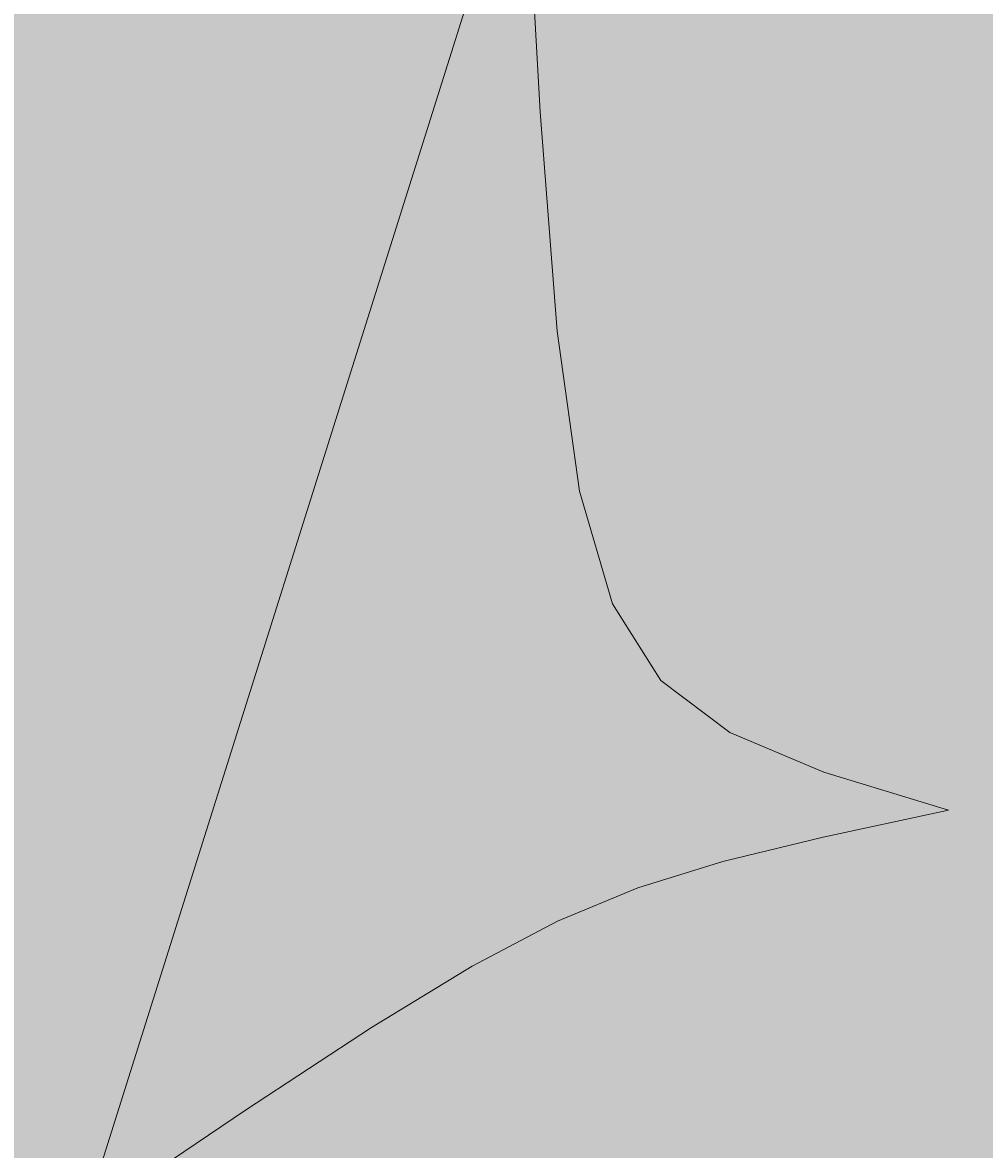
# Model space of a CAD drawing. Units: millimetres. Extents: x 27017497 to 27018854, y 7058029 to 7059154.
# Tile 84 of 91: x 27018341 to 27018362, y 7058530 to 7058555. Entities that reach past the tile are written whole.
import ezdxf

# ---------------------------------------------------------------- set-up
doc = ezdxf.new("R2010")
doc.units = ezdxf.units.MM
doc.layers.add('A-ANNO-DIMS', color=2, linetype='Continuous', lineweight=18)
doc.layers.add('A-FURN', color=8, linetype='Continuous', lineweight=18)
doc.layers.add('A-FURN-PATT', color=177, linetype='Continuous', lineweight=13, true_color=0x293189)
doc.styles.get("Standard").update_dxf_attribs({"font": 'arial.ttf'})
doc.dimstyles.get("Standard").update_dxf_attribs({"dimtxt": 0.18, "dimasz": 0.18, "dimexe": 0.18, "dimexo": 0.0625, "dimgap": 0.09, "dimtad": 0, "dimtih": 1, "dimtoh": 1, "dimdec": 4, "dimzin": 0, "dimdsep": 46, "dimtxsty": 'Standard', "dimcen": 0.09, "dimadec": 0, "dimazin": 0, "dimtfac": 1, "dimtdec": 4, "dimtofl": 0, "dimtmove": 0, "dimatfit": 3, "dimfxl": 1, "dimtolj": 1, "dimtzin": 0, "dimarcsym": 0})

# ---------------------------------------------------------------- blocks, each defined once
blk = doc.blocks.new('CAMMAT')
blk.add_line((0.05354, -0.5623), (-0.73116, -0.80928))
for points in [[(-0.17613, -1.04763), (-0.161, -0.97721), (-0.14737, -0.92096), (-0.13256, -0.87318), (-0.11386, -0.82818), (-0.0886, -0.78028), (-0.05407, -0.7238), (-0.00759, -0.65303), (0.05354, -0.5623)], [(-0.73116, -0.80928), (-0.56827, -0.81849), (-0.4451, -0.82799), (-0.35515, -0.84058), (-0.29193, -0.85906), (-0.24892, -0.8862), (-0.21962, -0.92482), (-0.19752, -0.9777), (-0.17613, -1.04763)]]:
    blk.add_lwpolyline(points)
blk = doc.blocks.new('*D48')
at = {"layer": 'A-ANNO-DIMS', "color": 0, "lineweight": -2, "transparency": 16777216}
for p, q in [((27018463.498, 7058622.912), (27017497.536, 7058622.912)), ((27017497.716, 7058622.732), (27017497.716, 7058357.753)), ((27017497.716, 7058092.41), (27017497.716, 7058357.389)), ((27018555.129, 7058092.23), (27017497.536, 7058092.23))]:
    blk.add_line(p, q, dxfattribs=at)
at = {"layer": 'A-ANNO-DIMS', "color": 0, "transparency": 16777216}
for points in [[(27017497.686, 7058622.732), (27017497.746, 7058622.732), (27017497.716, 7058622.912)], [(27017497.686, 7058092.41), (27017497.746, 7058092.41), (27017497.716, 7058092.23)]]:
    blk.add_solid(points, dxfattribs=at)
at = {"layer": 'Defpoints', "color": 0, "transparency": 16777216}
for p in [(27018463.561, 7058622.912), (27017497.716, 7058092.23), (27018555.192, 7058092.23)]:
    blk.add_point(p, dxfattribs=at)
at = {"layer": 'A-ANNO-DIMS', "color": 0, "transparency": 16777216, "insert": (27017497.716, 7058357.571), "char_height": 0.18, "attachment_point": 5}
blk.add_mtext('\\A1;530.7', dxfattribs=at)
blk = doc.blocks.new('*D50')
at = {"layer": 'A-ANNO-DIMS', "color": 0, "lineweight": -2, "transparency": 16777216}
for p, q in [((27018223.668, 7058580.912), (27018854.236, 7058580.912)), ((27018854.056, 7058580.732), (27018854.056, 7058511.344)), ((27018854.056, 7058441.592), (27018854.056, 7058510.98)), ((27018223.668, 7058441.412), (27018854.236, 7058441.412))]:
    blk.add_line(p, q, dxfattribs=at)
at = {"layer": 'A-ANNO-DIMS', "color": 0, "transparency": 16777216}
for points in [[(27018854.026, 7058580.732), (27018854.086, 7058580.732), (27018854.056, 7058580.912)], [(27018854.026, 7058441.592), (27018854.086, 7058441.592), (27018854.056, 7058441.412)]]:
    blk.add_solid(points, dxfattribs=at)
at = {"layer": 'Defpoints', "color": 0, "transparency": 16777216}
for p in [(27018223.606, 7058580.912), (27018223.606, 7058441.412), (27018854.056, 7058441.412)]:
    blk.add_point(p, dxfattribs=at)
at = {"layer": 'A-ANNO-DIMS', "color": 0, "transparency": 16777216, "insert": (27018854.056, 7058511.162), "char_height": 0.18, "attachment_point": 5}
blk.add_mtext('\\A1;139.5', dxfattribs=at)

msp = doc.modelspace()

# ---------------------------------------------------------------- hatches: boundary and pattern name
at = {"layer": 'A-FURN-PATT'}
h = msp.add_hatch(color=256, dxfattribs=at)
h.dxf.hatch_style = 1
h.paths.add_polyline_path([(27018398.067, 7058554.497, 0.414214), (27018396.474, 7058556.09), (27018352.018, 7058556.09), (27018352.202, 7058552.834), (27018352.581, 7058547.929), (27018353.082, 7058544.346), (27018353.818, 7058541.828), (27018354.899, 7058540.115), (27018356.437, 7058538.948), (27018358.543, 7058538.068), (27018361.329, 7058537.215), (27018358.524, 7058536.613), (27018356.284, 7058536.07), (27018354.381, 7058535.48), (27018352.588, 7058534.736), (27018350.68, 7058533.729), (27018348.431, 7058532.354), (27018345.612, 7058530.503), (27018341.998, 7058528.068), (27018345.612, 7058525.633), (27018348.431, 7058523.782), (27018350.68, 7058522.407), (27018352.588, 7058521.4), (27018354.381, 7058520.656), (27018356.284, 7058520.066), (27018358.524, 7058519.523), (27018361.329, 7058518.92), (27018358.543, 7058518.068), (27018356.437, 7058517.188), (27018354.899, 7058516.021), (27018353.818, 7058514.308), (27018353.082, 7058511.79), (27018352.581, 7058508.207), (27018352.28, 7058504.311), (27018396.474, 7058504.311, 0.414214), (27018398.067, 7058505.904)])
h.paths.add_polyline_path([(27018356.437, 7058538.948), (27018354.899, 7058540.115), (27018353.818, 7058541.828), (27018353.082, 7058544.346), (27018352.581, 7058547.929), (27018352.202, 7058552.834), (27018351.835, 7058559.322), (27018341.998, 7058528.068), (27018345.612, 7058530.503), (27018348.431, 7058532.354), (27018350.68, 7058533.729), (27018352.588, 7058534.736), (27018354.381, 7058535.48), (27018356.284, 7058536.07), (27018358.524, 7058536.613), (27018361.329, 7058537.215), (27018358.543, 7058538.068)])
h.paths.add_polyline_path([(27018358.543, 7058518.068), (27018361.329, 7058518.92), (27018358.524, 7058519.523), (27018356.284, 7058520.066), (27018354.381, 7058520.656), (27018352.588, 7058521.4), (27018350.68, 7058522.407), (27018348.431, 7058523.782), (27018345.612, 7058525.633), (27018341.998, 7058528.068), (27018351.835, 7058496.813), (27018352.202, 7058503.301), (27018352.581, 7058508.207), (27018353.082, 7058511.79), (27018353.818, 7058514.308), (27018354.899, 7058516.021), (27018356.437, 7058517.188)])
h.paths.add_polyline_path([(27018351.324, 7058557.699), (27018340.191, 7058557.699), (27018340.191, 7058503.014), (27018349.884, 7058503.014), (27018341.998, 7058528.068)])
h.paths.add_polyline_path([(27018340.191, 7058556.09), (27018323.983, 7058556.09, 0.414214), (27018322.39, 7058554.497), (27018322.39, 7058505.904, 0.414214), (27018323.983, 7058504.311), (27018340.191, 7058504.311)])
h.paths.add_polyline_path([(27018337.107, 7058532.051, -0.414214), (27018335.912, 7058530.856), (27018326.353, 7058530.856, -0.414214), (27018325.158, 7058532.051), (27018325.158, 7058553.51, -0.414214), (27018326.353, 7058554.705), (27018335.912, 7058554.705, -0.414214), (27018337.107, 7058553.51)], flags=0)
h.paths.add_polyline_path([(27018337.107, 7058527.914), (27018337.107, 7058506.454, -0.414214), (27018335.912, 7058505.259), (27018326.353, 7058505.259, -0.414214), (27018325.158, 7058506.454), (27018325.158, 7058527.914, -0.414214), (27018326.353, 7058529.109), (27018335.912, 7058529.109, -0.414214)], flags=0)
h.paths.add_polyline_path([(27018338.322, 7058577.2), (27018322.39, 7058577.2), (27018322.39, 7058557.285), (27018338.322, 7058557.285)])
h.paths.add_polyline_path([(27018323.748, 7058567.284, -1), (27018335.697, 7058567.284, -1)], flags=16)
h.paths.add_polyline_path([(27018326.023, 7058567.284, -1), (27018333.423, 7058567.284, -1)], flags=0)
h.paths.add_polyline_path([(27018338.322, 7058503.116), (27018322.39, 7058503.116), (27018322.39, 7058483.201), (27018338.322, 7058483.201)])
h.paths.add_polyline_path([(27018335.697, 7058493.391, -1), (27018323.748, 7058493.391, -1)], flags=16)
h.paths.add_polyline_path([(27018333.423, 7058493.391, -1), (27018326.023, 7058493.391, -1)], flags=0)
h.paths.add_polyline_path([(27018337.107, 7058527.914, 0.414214), (27018335.912, 7058529.109), (27018326.353, 7058529.109, 0.414214), (27018325.158, 7058527.914), (27018325.158, 7058506.454, 0.414214), (27018326.353, 7058505.259), (27018335.912, 7058505.259, 0.414214), (27018337.107, 7058506.454)], flags=16)
h.paths.add_polyline_path([(27018337.107, 7058553.51, 0.414214), (27018335.912, 7058554.705), (27018326.353, 7058554.705, 0.414214), (27018325.158, 7058553.51), (27018325.158, 7058532.051, 0.414214), (27018326.353, 7058530.856), (27018335.912, 7058530.856, 0.414214), (27018337.107, 7058532.051)], flags=16)

# ---------------------------------------------------------------- block references
at = {"layer": 'A-FURN', "xscale": -39.82996475819422, "yscale": 39.82996475819422, "zscale": 39.82996475819422, "rotation": 90}
msp.add_blockref('CAMMAT', (27018319.602, 7058530.2), dxfattribs=at)

# ---------------------------------------------------------------- dimensions: what is measured, and where the dimension line sits
at = {"layer": 'A-ANNO-DIMS'}
for base, p1, p2, picture, middle in [((27017497.716, 7058092.23), (27018463.561, 7058622.912), (27018555.192, 7058092.23), '*D48', (27017497.716, 7058357.571)), ((27018854.056, 7058441.412), (27018223.606, 7058580.912), (27018223.606, 7058441.412), '*D50', (27018854.056, 7058511.162))]:
    dim = msp.add_linear_dim(base=base, p1=p1, p2=p2, angle=90, dimstyle='Standard', override={"dimdec": 1, "dimlfac": 1, "dimrnd": 0, "dimzin": 0, "dimdsep": 46, "dimlunit": 2}, dxfattribs=at)
    dim.commit()
    dim.dimension.update_dxf_attribs({"geometry": picture, "text_midpoint": middle})

doc.saveas('drawing.dxf')
